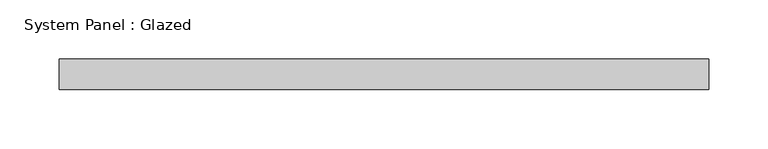
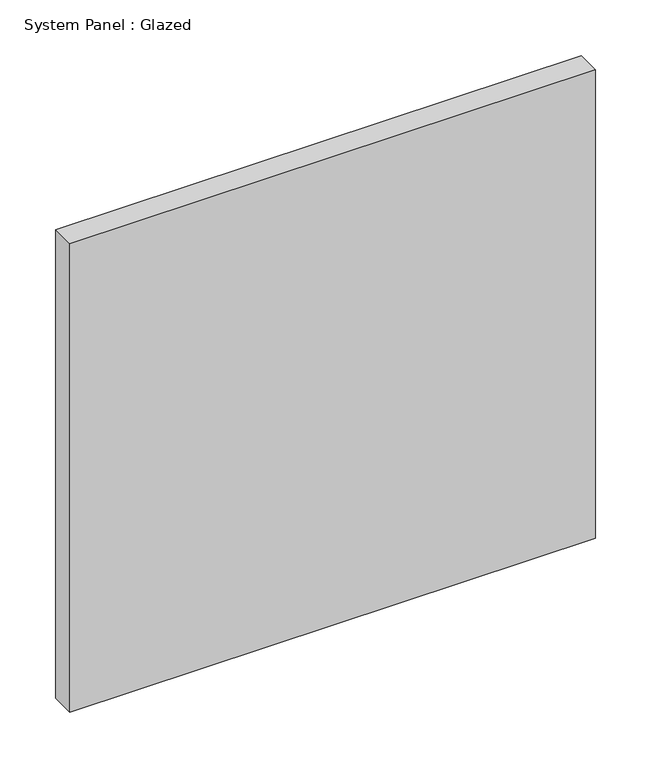
"""IFC4 building model written with IfcOpenShell, lengths in millimetres: plate geometry, System Panel : Glazed."""

from ifc_helpers import new_model, si_unit, origin, origin_with_axes, place, context, project, spatial, polyline, outline, extrude, source, transform, mapped, element, save


def system_panel_glazed_4278ab3a(model_context):
    return source(origin(), model_context, "Body", "SweptSolid", [
        extrude(outline(polyline([(273.05, 19.05), (-273.05, 19.05), (-273.05, 44.45), (273.05, 44.45), (273.05, 19.05)])), origin_with_axes(), (0.0, 0.0, 1.0), 514.35),
    ])


if __name__ == "__main__":
    model = new_model("IFC4")
    model_context = context("Model", 3, world=origin())
    ifc_project = project(units=[si_unit("LENGTHUNIT", "METRE", prefix="MILLI")], contexts=[model_context])
    site = spatial("IfcSite", under=ifc_project)
    building = spatial("IfcBuilding", under=site)
    placement = place(None, origin())
    system_panel_glazed_shape = system_panel_glazed_4278ab3a(model_context)
    element("IfcPlate", 1, ObjectType="System Panel : Glazed", at=placement, inside=building, context=model_context, shape_type="MappedRepresentation", body=[
        mapped(system_panel_glazed_shape, transform((0.0, 0.0, 0.0), x_axis=(1.0, 0.0, 0.0), y_axis=(0.0, 1.0, 0.0), z_axis=(0.0, 0.0, 1.0))),
    ])
    save(model, "model.ifc")

# Revit data of these elements
# Type "System Panel : Glazed"
#   Construction Type Id = "GSP4R"
#   Analytic Construction = "1/8 in Pilkington single glazing"
#   Visual Light Transmittance = 0.9
#   Solar Heat Gain Coefficient = 0.86
#   Heat Transfer Coefficient (U) = 1.18115 BTU/(h·ft²·°F)
#   Define Thermal Properties by = 1
# Element 1 (IfcPlate, "System Panel : Glazed")
#   Materials on its faces: "Glass"
# Materials
#   "Glass": class "Glass", colour RGB 0 128 192, transparency 0.75, Description = "Soda Lime Glass", Cost = 0
